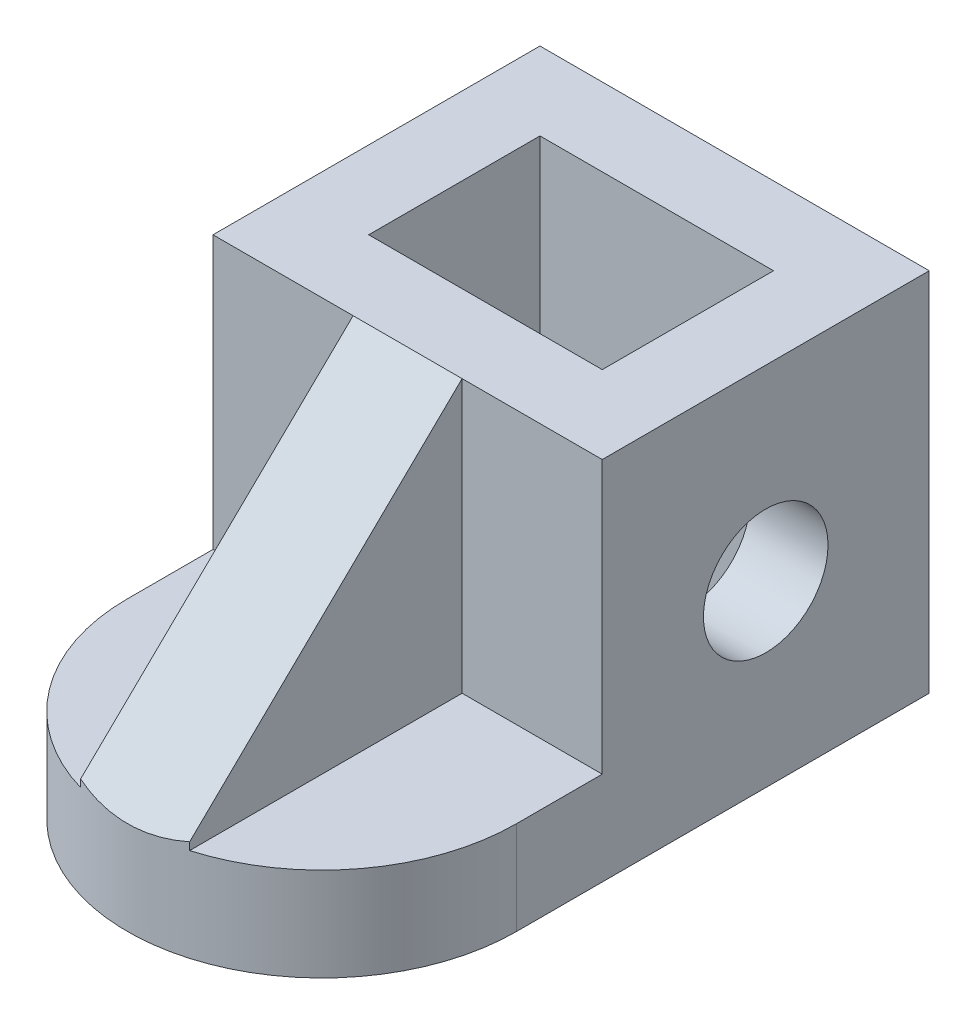
ISO-10303-21;
HEADER;
FILE_DESCRIPTION(('STEP AP214'),'2;1');
FILE_NAME('part.step','',(''),(''),'','','');
FILE_SCHEMA(('AUTOMOTIVE_DESIGN { 1 0 10303 214 1 1 1 1 }'));
ENDSEC;
DATA;
#1=APPLICATION_CONTEXT('core data for automotive mechanical design processes');
#2=APPLICATION_PROTOCOL_DEFINITION('international standard','automotive_design',2000,#1);
#3=PRODUCT_CONTEXT('',#1,'mechanical');
#4=PRODUCT('Part','Part','',(#3));
#5=PRODUCT_RELATED_PRODUCT_CATEGORY('part','',(#4));
#6=PRODUCT_DEFINITION_FORMATION('','',#4);
#7=PRODUCT_DEFINITION_CONTEXT('part definition',#1,'design');
#8=PRODUCT_DEFINITION('design','',#6,#7);
#9=PRODUCT_DEFINITION_SHAPE('','',#8);
#10=(LENGTH_UNIT() NAMED_UNIT(*) SI_UNIT(.MILLI.,.METRE.));
#11=(NAMED_UNIT(*) PLANE_ANGLE_UNIT() SI_UNIT($,.RADIAN.));
#12=(NAMED_UNIT(*) SI_UNIT($,.STERADIAN.) SOLID_ANGLE_UNIT());
#13=UNCERTAINTY_MEASURE_WITH_UNIT(LENGTH_MEASURE(1.E-05),#10,'distance_accuracy_value','');
#14=(GEOMETRIC_REPRESENTATION_CONTEXT(3) GLOBAL_UNCERTAINTY_ASSIGNED_CONTEXT((#13)) GLOBAL_UNIT_ASSIGNED_CONTEXT((#10,
#11,#12)) REPRESENTATION_CONTEXT('',''));
#15=CARTESIAN_POINT('',(0.,0.,0.));
#16=DIRECTION('',(0.,0.,1.));
#17=DIRECTION('',(1.,0.,0.));
#18=AXIS2_PLACEMENT_3D('',#15,#16,#17);
#19=CARTESIAN_POINT('',(-25.,6.,39.));
#20=DIRECTION('',(0.,-0.716994918814431,-0.697078393291808));
#21=DIRECTION('',(0.,0.697078393291808,-0.716994918814431));
#22=AXIS2_PLACEMENT_3D('',#19,#20,#21);
#23=PLANE('',#22);
#24=DIRECTION('',(0.,0.697078393291808,-0.716994918814431));
#25=VECTOR('',#24,1.);
#26=CARTESIAN_POINT('',(-32.,6.,39.));
#27=LINE('',#26,#25);
#28=CARTESIAN_POINT('',(-32.,6.97222222222222,38.));
#29=VERTEX_POINT('',#28);
#30=CARTESIAN_POINT('',(-32.,41.,3.00000000000002));
#31=VERTEX_POINT('',#30);
#32=EDGE_CURVE('E158',#29,#31,#27,.T.);
#33=ORIENTED_EDGE('',*,*,#32,.F.);
#34=CARTESIAN_POINT('',(-25.,30.3055555555556,14.));
#35=DIRECTION('',(0.,-0.716994918814431,-0.697078393291808));
#36=DIRECTION('',(0.,-0.697078393291808,0.716994918814431));
#37=AXIS2_PLACEMENT_3D('',#34,#35,#36);
#38=ELLIPSE('',#37,34.8677505850922,25.);
#39=CARTESIAN_POINT('',(-18.,6.97222222222222,38.));
#40=VERTEX_POINT('',#39);
#41=EDGE_CURVE('E145',#29,#40,#38,.F.);
#42=ORIENTED_EDGE('',*,*,#41,.T.);
#43=DIRECTION('',(0.,0.697078393291808,-0.716994918814431));
#44=VECTOR('',#43,1.);
#45=CARTESIAN_POINT('',(-18.,6.,39.));
#46=LINE('',#45,#44);
#47=CARTESIAN_POINT('',(-18.,41.,3.00000000000003));
#48=VERTEX_POINT('',#47);
#49=EDGE_CURVE('E53',#40,#48,#46,.T.);
#50=ORIENTED_EDGE('',*,*,#49,.T.);
#51=DIRECTION('',(1.,0.,0.));
#52=VECTOR('',#51,1.);
#53=CARTESIAN_POINT('',(-50.,41.,3.00000000000003));
#54=LINE('',#53,#52);
#55=EDGE_CURVE('E156',#31,#48,#54,.T.);
#56=ORIENTED_EDGE('',*,*,#55,.F.);
#57=EDGE_LOOP('',(#33,#42,#50,#56));
#58=FACE_BOUND('',#57,.T.);
#59=ADVANCED_FACE('F39',(#58),#23,.F.);
#60=CARTESIAN_POINT('',(-32.,17.5,0.));
#61=DIRECTION('',(1.,0.,0.));
#62=DIRECTION('',(0.,0.,-1.));
#63=AXIS2_PLACEMENT_3D('',#60,#61,#62);
#64=PLANE('',#63);
#65=DIRECTION('',(0.,-1.,0.));
#66=VECTOR('',#65,1.);
#67=CARTESIAN_POINT('',(-32.,14.,38.));
#68=LINE('',#67,#66);
#69=CARTESIAN_POINT('',(-32.,6.,38.));
#70=VERTEX_POINT('',#69);
#71=EDGE_CURVE('E143',#29,#70,#68,.T.);
#72=ORIENTED_EDGE('',*,*,#71,.F.);
#73=ORIENTED_EDGE('',*,*,#32,.T.);
#74=DIRECTION('',(0.,1.,0.));
#75=VECTOR('',#74,1.);
#76=CARTESIAN_POINT('',(-32.,5.99999999999999,3.00000000000003));
#77=LINE('',#76,#75);
#78=CARTESIAN_POINT('',(-32.,5.99999999999999,3.00000000000003));
#79=VERTEX_POINT('',#78);
#80=EDGE_CURVE('E165',#79,#31,#77,.T.);
#81=ORIENTED_EDGE('',*,*,#80,.F.);
#82=DIRECTION('',(0.,0.,-1.));
#83=VECTOR('',#82,1.);
#84=CARTESIAN_POINT('',(-32.,6.,39.));
#85=LINE('',#84,#83);
#86=EDGE_CURVE('E159',#70,#79,#85,.T.);
#87=ORIENTED_EDGE('',*,*,#86,.F.);
#88=EDGE_LOOP('',(#72,#73,#81,#87));
#89=FACE_BOUND('',#88,.T.);
#90=ADVANCED_FACE('F151',(#89),#64,.F.);
#91=CARTESIAN_POINT('',(-50.,-6.,39.));
#92=DIRECTION('',(0.,-1.,0.));
#93=DIRECTION('',(0.,0.,-1.));
#94=AXIS2_PLACEMENT_3D('',#91,#92,#93);
#95=PLANE('',#94);
#96=DIRECTION('',(-1.,0.,0.));
#97=VECTOR('',#96,1.);
#98=CARTESIAN_POINT('',(-40.,-6.,-29.));
#99=LINE('',#98,#97);
#100=CARTESIAN_POINT('',(-10.,-6.,-29.));
#101=VERTEX_POINT('',#100);
#102=CARTESIAN_POINT('',(-40.,-6.,-29.));
#103=VERTEX_POINT('',#102);
#104=EDGE_CURVE('E61',#101,#103,#99,.T.);
#105=ORIENTED_EDGE('',*,*,#104,.T.);
#106=DIRECTION('',(0.,0.,1.));
#107=VECTOR('',#106,1.);
#108=CARTESIAN_POINT('',(-40.,-6.,-29.));
#109=LINE('',#108,#107);
#110=CARTESIAN_POINT('',(-40.,-6.00000000000001,-6.99999999999997));
#111=VERTEX_POINT('',#110);
#112=EDGE_CURVE('E193',#103,#111,#109,.T.);
#113=ORIENTED_EDGE('',*,*,#112,.T.);
#114=DIRECTION('',(1.,0.,0.));
#115=VECTOR('',#114,1.);
#116=CARTESIAN_POINT('',(-40.,-6.00000000000001,-6.99999999999997));
#117=LINE('',#116,#115);
#118=CARTESIAN_POINT('',(-10.,-6.00000000000001,-6.99999999999997));
#119=VERTEX_POINT('',#118);
#120=EDGE_CURVE('E197',#111,#119,#117,.T.);
#121=ORIENTED_EDGE('',*,*,#120,.T.);
#122=DIRECTION('',(0.,0.,-1.));
#123=VECTOR('',#122,1.);
#124=CARTESIAN_POINT('',(-10.,-6.,-29.));
#125=LINE('',#124,#123);
#126=EDGE_CURVE('E188',#119,#101,#125,.T.);
#127=ORIENTED_EDGE('',*,*,#126,.T.);
#128=EDGE_LOOP('',(#105,#113,#121,#127));
#129=FACE_BOUND('',#128,.T.);
#130=DIRECTION('',(0.,0.,-1.));
#131=VECTOR('',#130,1.);
#132=CARTESIAN_POINT('',(0.,-6.,39.));
#133=LINE('',#132,#131);
#134=CARTESIAN_POINT('',(0.,-6.00000000000001,14.));
#135=VERTEX_POINT('',#134);
#136=CARTESIAN_POINT('',(0.,-6.,-39.));
#137=VERTEX_POINT('',#136);
#138=EDGE_CURVE('E245',#135,#137,#133,.T.);
#139=ORIENTED_EDGE('',*,*,#138,.F.);
#140=CARTESIAN_POINT('',(-25.,-6.00000000000001,14.));
#141=DIRECTION('',(0.,1.,0.));
#142=DIRECTION('',(0.,0.,1.));
#143=AXIS2_PLACEMENT_3D('',#140,#141,#142);
#144=CIRCLE('',#143,25.);
#145=CARTESIAN_POINT('',(-50.,-6.00000000000001,14.));
#146=VERTEX_POINT('',#145);
#147=EDGE_CURVE('E170',#146,#135,#144,.T.);
#148=ORIENTED_EDGE('',*,*,#147,.F.);
#149=DIRECTION('',(0.,0.,-1.));
#150=VECTOR('',#149,1.);
#151=CARTESIAN_POINT('',(-50.,-6.,39.));
#152=LINE('',#151,#150);
#153=CARTESIAN_POINT('',(-50.,-6.,-39.));
#154=VERTEX_POINT('',#153);
#155=EDGE_CURVE('E50',#146,#154,#152,.T.);
#156=ORIENTED_EDGE('',*,*,#155,.T.);
#157=DIRECTION('',(1.,0.,0.));
#158=VECTOR('',#157,1.);
#159=CARTESIAN_POINT('',(-50.,-6.,-39.));
#160=LINE('',#159,#158);
#161=EDGE_CURVE('E11',#154,#137,#160,.T.);
#162=ORIENTED_EDGE('',*,*,#161,.T.);
#163=EDGE_LOOP('',(#139,#148,#156,#162));
#164=FACE_BOUND('',#163,.T.);
#165=ADVANCED_FACE('F257',(#129,#164),#95,.T.);
#166=CARTESIAN_POINT('',(-18.,17.5,0.));
#167=DIRECTION('',(1.,0.,0.));
#168=DIRECTION('',(0.,0.,-1.));
#169=AXIS2_PLACEMENT_3D('',#166,#167,#168);
#170=PLANE('',#169);
#171=ORIENTED_EDGE('',*,*,#49,.F.);
#172=DIRECTION('',(0.,-1.,0.));
#173=VECTOR('',#172,1.);
#174=CARTESIAN_POINT('',(-18.,14.,38.));
#175=LINE('',#174,#173);
#176=CARTESIAN_POINT('',(-18.,6.,38.));
#177=VERTEX_POINT('',#176);
#178=EDGE_CURVE('E150',#40,#177,#175,.T.);
#179=ORIENTED_EDGE('',*,*,#178,.T.);
#180=DIRECTION('',(0.,0.,-1.));
#181=VECTOR('',#180,1.);
#182=CARTESIAN_POINT('',(-18.,6.,39.));
#183=LINE('',#182,#181);
#184=CARTESIAN_POINT('',(-18.,5.99999999999999,3.00000000000003));
#185=VERTEX_POINT('',#184);
#186=EDGE_CURVE('E174',#177,#185,#183,.T.);
#187=ORIENTED_EDGE('',*,*,#186,.T.);
#188=DIRECTION('',(0.,1.,0.));
#189=VECTOR('',#188,1.);
#190=CARTESIAN_POINT('',(-18.,5.99999999999999,3.00000000000003));
#191=LINE('',#190,#189);
#192=EDGE_CURVE('E173',#185,#48,#191,.T.);
#193=ORIENTED_EDGE('',*,*,#192,.T.);
#194=EDGE_LOOP('',(#171,#179,#187,#193));
#195=FACE_BOUND('',#194,.T.);
#196=ADVANCED_FACE('F293',(#195),#170,.T.);
#197=CARTESIAN_POINT('',(-50.,6.,39.));
#198=DIRECTION('',(0.,1.,0.));
#199=DIRECTION('',(0.,0.,1.));
#200=AXIS2_PLACEMENT_3D('',#197,#198,#199);
#201=PLANE('',#200);
#202=DIRECTION('',(0.,0.,1.));
#203=VECTOR('',#202,1.);
#204=CARTESIAN_POINT('',(-50.,6.,39.));
#205=LINE('',#204,#203);
#206=CARTESIAN_POINT('',(-50.,6.,3.00000000000003));
#207=VERTEX_POINT('',#206);
#208=CARTESIAN_POINT('',(-50.,6.,14.));
#209=VERTEX_POINT('',#208);
#210=EDGE_CURVE('E241',#207,#209,#205,.T.);
#211=ORIENTED_EDGE('',*,*,#210,.T.);
#212=CARTESIAN_POINT('',(-25.,6.,14.));
#213=DIRECTION('',(0.,1.,0.));
#214=DIRECTION('',(0.,0.,1.));
#215=AXIS2_PLACEMENT_3D('',#212,#213,#214);
#216=CIRCLE('',#215,25.);
#217=EDGE_CURVE('E288',#209,#70,#216,.T.);
#218=ORIENTED_EDGE('',*,*,#217,.T.);
#219=ORIENTED_EDGE('',*,*,#86,.T.);
#220=DIRECTION('',(1.,0.,0.));
#221=VECTOR('',#220,1.);
#222=CARTESIAN_POINT('',(-50.,5.99999999999999,3.00000000000003));
#223=LINE('',#222,#221);
#224=EDGE_CURVE('E230',#207,#79,#223,.T.);
#225=ORIENTED_EDGE('',*,*,#224,.F.);
#226=EDGE_LOOP('',(#211,#218,#219,#225));
#227=FACE_BOUND('',#226,.T.);
#228=ADVANCED_FACE('F291',(#227),#201,.T.);
#229=ORIENTED_EDGE('',*,*,#186,.F.);
#230=CARTESIAN_POINT('',(-25.,6.,14.));
#231=DIRECTION('',(0.,1.,0.));
#232=DIRECTION('',(0.,0.,1.));
#233=AXIS2_PLACEMENT_3D('',#230,#231,#232);
#234=CIRCLE('',#233,25.);
#235=CARTESIAN_POINT('',(0.,6.,14.));
#236=VERTEX_POINT('',#235);
#237=EDGE_CURVE('E147',#177,#236,#234,.T.);
#238=ORIENTED_EDGE('',*,*,#237,.T.);
#239=DIRECTION('',(0.,0.,1.));
#240=VECTOR('',#239,1.);
#241=CARTESIAN_POINT('',(0.,6.,39.));
#242=LINE('',#241,#240);
#243=CARTESIAN_POINT('',(0.,5.99999999999999,3.00000000000003));
#244=VERTEX_POINT('',#243);
#245=EDGE_CURVE('E247',#244,#236,#242,.T.);
#246=ORIENTED_EDGE('',*,*,#245,.F.);
#247=EDGE_CURVE('E231',#185,#244,#223,.T.);
#248=ORIENTED_EDGE('',*,*,#247,.F.);
#249=EDGE_LOOP('',(#229,#238,#246,#248));
#250=FACE_BOUND('',#249,.T.);
#251=ADVANCED_FACE('F281',(#250),#201,.T.);
#252=CARTESIAN_POINT('',(-50.,0.,0.));
#253=DIRECTION('',(-1.,0.,0.));
#254=DIRECTION('',(0.,0.,1.));
#255=AXIS2_PLACEMENT_3D('',#252,#253,#254);
#256=PLANE('',#255);
#257=CARTESIAN_POINT('',(-50.,17.,-18.));
#258=DIRECTION('',(-1.,0.,0.));
#259=DIRECTION('',(0.,0.,1.));
#260=AXIS2_PLACEMENT_3D('',#257,#258,#259);
#261=CIRCLE('',#260,8.);
#262=CARTESIAN_POINT('',(-50.,17.,-9.99999999999997));
#263=VERTEX_POINT('',#262);
#264=EDGE_CURVE('E180',#263,#263,#261,.T.);
#265=ORIENTED_EDGE('',*,*,#264,.F.);
#266=EDGE_LOOP('',(#265));
#267=FACE_BOUND('',#266,.T.);
#268=ORIENTED_EDGE('',*,*,#155,.F.);
#269=DIRECTION('',(0.,1.,0.));
#270=VECTOR('',#269,1.);
#271=CARTESIAN_POINT('',(-50.,-6.00000000000001,14.));
#272=LINE('',#271,#270);
#273=EDGE_CURVE('E162',#146,#209,#272,.T.);
#274=ORIENTED_EDGE('',*,*,#273,.T.);
#275=ORIENTED_EDGE('',*,*,#210,.F.);
#276=DIRECTION('',(0.,-1.,0.));
#277=VECTOR('',#276,1.);
#278=CARTESIAN_POINT('',(-50.,5.99999999999999,3.00000000000003));
#279=LINE('',#278,#277);
#280=CARTESIAN_POINT('',(-50.,41.,3.00000000000003));
#281=VERTEX_POINT('',#280);
#282=EDGE_CURVE('E218',#281,#207,#279,.T.);
#283=ORIENTED_EDGE('',*,*,#282,.F.);
#284=DIRECTION('',(0.,0.,1.));
#285=VECTOR('',#284,1.);
#286=CARTESIAN_POINT('',(-50.,41.,-39.));
#287=LINE('',#286,#285);
#288=CARTESIAN_POINT('',(-50.,41.,-39.));
#289=VERTEX_POINT('',#288);
#290=EDGE_CURVE('E220',#289,#281,#287,.T.);
#291=ORIENTED_EDGE('',*,*,#290,.F.);
#292=DIRECTION('',(0.,1.,0.));
#293=VECTOR('',#292,1.);
#294=CARTESIAN_POINT('',(-50.,-6.,-39.));
#295=LINE('',#294,#293);
#296=EDGE_CURVE('E237',#154,#289,#295,.T.);
#297=ORIENTED_EDGE('',*,*,#296,.F.);
#298=EDGE_LOOP('',(#268,#274,#275,#283,#291,#297));
#299=FACE_BOUND('',#298,.T.);
#300=ADVANCED_FACE('F266',(#267,#299),#256,.T.);
#301=CARTESIAN_POINT('',(0.,0.,0.));
#302=DIRECTION('',(-1.,0.,0.));
#303=DIRECTION('',(0.,0.,1.));
#304=AXIS2_PLACEMENT_3D('',#301,#302,#303);
#305=PLANE('',#304);
#306=CARTESIAN_POINT('',(0.,17.,-18.));
#307=DIRECTION('',(1.,0.,0.));
#308=DIRECTION('',(0.,0.,-1.));
#309=AXIS2_PLACEMENT_3D('',#306,#307,#308);
#310=CIRCLE('',#309,8.);
#311=CARTESIAN_POINT('',(0.,17.,-26.));
#312=VERTEX_POINT('',#311);
#313=EDGE_CURVE('E181',#312,#312,#310,.T.);
#314=ORIENTED_EDGE('',*,*,#313,.F.);
#315=EDGE_LOOP('',(#314));
#316=FACE_BOUND('',#315,.T.);
#317=DIRECTION('',(0.,1.,0.));
#318=VECTOR('',#317,1.);
#319=CARTESIAN_POINT('',(0.,-6.00000000000001,14.));
#320=LINE('',#319,#318);
#321=EDGE_CURVE('E259',#135,#236,#320,.T.);
#322=ORIENTED_EDGE('',*,*,#321,.F.);
#323=ORIENTED_EDGE('',*,*,#138,.T.);
#324=DIRECTION('',(0.,1.,0.));
#325=VECTOR('',#324,1.);
#326=CARTESIAN_POINT('',(0.,-6.,-39.));
#327=LINE('',#326,#325);
#328=CARTESIAN_POINT('',(0.,41.,-39.));
#329=VERTEX_POINT('',#328);
#330=EDGE_CURVE('E235',#137,#329,#327,.T.);
#331=ORIENTED_EDGE('',*,*,#330,.T.);
#332=DIRECTION('',(0.,0.,1.));
#333=VECTOR('',#332,1.);
#334=CARTESIAN_POINT('',(0.,41.,-39.));
#335=LINE('',#334,#333);
#336=CARTESIAN_POINT('',(0.,41.,3.00000000000003));
#337=VERTEX_POINT('',#336);
#338=EDGE_CURVE('E209',#329,#337,#335,.T.);
#339=ORIENTED_EDGE('',*,*,#338,.T.);
#340=DIRECTION('',(0.,-1.,0.));
#341=VECTOR('',#340,1.);
#342=CARTESIAN_POINT('',(0.,5.99999999999999,3.00000000000003));
#343=LINE('',#342,#341);
#344=EDGE_CURVE('E223',#337,#244,#343,.T.);
#345=ORIENTED_EDGE('',*,*,#344,.T.);
#346=ORIENTED_EDGE('',*,*,#245,.T.);
#347=EDGE_LOOP('',(#322,#323,#331,#339,#345,#346));
#348=FACE_BOUND('',#347,.T.);
#349=ADVANCED_FACE('F254',(#316,#348),#305,.F.);
#350=CARTESIAN_POINT('',(-50.,5.99999999999999,3.00000000000003));
#351=DIRECTION('',(0.,0.,1.));
#352=DIRECTION('',(0.,-1.,0.));
#353=AXIS2_PLACEMENT_3D('',#350,#351,#352);
#354=PLANE('',#353);
#355=ORIENTED_EDGE('',*,*,#224,.T.);
#356=ORIENTED_EDGE('',*,*,#80,.T.);
#357=EDGE_CURVE('E234',#281,#31,#54,.T.);
#358=ORIENTED_EDGE('',*,*,#357,.F.);
#359=ORIENTED_EDGE('',*,*,#282,.T.);
#360=EDGE_LOOP('',(#355,#356,#358,#359));
#361=FACE_BOUND('',#360,.T.);
#362=ADVANCED_FACE('F271',(#361),#354,.T.);
#363=CARTESIAN_POINT('',(-50.,-6.,-39.));
#364=DIRECTION('',(0.,0.,-1.));
#365=DIRECTION('',(-1.,0.,0.));
#366=AXIS2_PLACEMENT_3D('',#363,#364,#365);
#367=PLANE('',#366);
#368=ORIENTED_EDGE('',*,*,#330,.F.);
#369=ORIENTED_EDGE('',*,*,#161,.F.);
#370=ORIENTED_EDGE('',*,*,#296,.T.);
#371=DIRECTION('',(1.,0.,0.));
#372=VECTOR('',#371,1.);
#373=CARTESIAN_POINT('',(-50.,41.,-39.));
#374=LINE('',#373,#372);
#375=EDGE_CURVE('E225',#289,#329,#374,.T.);
#376=ORIENTED_EDGE('',*,*,#375,.T.);
#377=EDGE_LOOP('',(#368,#369,#370,#376));
#378=FACE_BOUND('',#377,.T.);
#379=ADVANCED_FACE('F41',(#378),#367,.T.);
#380=ORIENTED_EDGE('',*,*,#192,.F.);
#381=ORIENTED_EDGE('',*,*,#247,.T.);
#382=ORIENTED_EDGE('',*,*,#344,.F.);
#383=EDGE_CURVE('E240',#48,#337,#54,.T.);
#384=ORIENTED_EDGE('',*,*,#383,.F.);
#385=EDGE_LOOP('',(#380,#381,#382,#384));
#386=FACE_BOUND('',#385,.T.);
#387=ADVANCED_FACE('F280',(#386),#354,.T.);
#388=CARTESIAN_POINT('',(-50.,41.,-39.));
#389=DIRECTION('',(0.,1.,0.));
#390=DIRECTION('',(0.,0.,1.));
#391=AXIS2_PLACEMENT_3D('',#388,#389,#390);
#392=PLANE('',#391);
#393=DIRECTION('',(0.,0.,-1.));
#394=VECTOR('',#393,1.);
#395=CARTESIAN_POINT('',(-10.,41.,-29.));
#396=LINE('',#395,#394);
#397=CARTESIAN_POINT('',(-10.,41.,-6.99999999999996));
#398=VERTEX_POINT('',#397);
#399=CARTESIAN_POINT('',(-10.,41.,-29.));
#400=VERTEX_POINT('',#399);
#401=EDGE_CURVE('E190',#398,#400,#396,.T.);
#402=ORIENTED_EDGE('',*,*,#401,.F.);
#403=DIRECTION('',(1.,0.,0.));
#404=VECTOR('',#403,1.);
#405=CARTESIAN_POINT('',(-40.,41.,-6.99999999999996));
#406=LINE('',#405,#404);
#407=CARTESIAN_POINT('',(-40.,41.,-6.99999999999996));
#408=VERTEX_POINT('',#407);
#409=EDGE_CURVE('E191',#408,#398,#406,.T.);
#410=ORIENTED_EDGE('',*,*,#409,.F.);
#411=DIRECTION('',(0.,0.,1.));
#412=VECTOR('',#411,1.);
#413=CARTESIAN_POINT('',(-40.,41.,-29.));
#414=LINE('',#413,#412);
#415=CARTESIAN_POINT('',(-40.,41.,-29.));
#416=VERTEX_POINT('',#415);
#417=EDGE_CURVE('E204',#416,#408,#414,.T.);
#418=ORIENTED_EDGE('',*,*,#417,.F.);
#419=DIRECTION('',(-1.,0.,0.));
#420=VECTOR('',#419,1.);
#421=CARTESIAN_POINT('',(-40.,41.,-29.));
#422=LINE('',#421,#420);
#423=EDGE_CURVE('E198',#400,#416,#422,.T.);
#424=ORIENTED_EDGE('',*,*,#423,.F.);
#425=EDGE_LOOP('',(#402,#410,#418,#424));
#426=FACE_BOUND('',#425,.T.);
#427=ORIENTED_EDGE('',*,*,#55,.T.);
#428=ORIENTED_EDGE('',*,*,#383,.T.);
#429=ORIENTED_EDGE('',*,*,#338,.F.);
#430=ORIENTED_EDGE('',*,*,#375,.F.);
#431=ORIENTED_EDGE('',*,*,#290,.T.);
#432=ORIENTED_EDGE('',*,*,#357,.T.);
#433=EDGE_LOOP('',(#427,#428,#429,#430,#431,#432));
#434=FACE_BOUND('',#433,.T.);
#435=ADVANCED_FACE('F269',(#426,#434),#392,.T.);
#436=CARTESIAN_POINT('',(-10.,-6.,-29.));
#437=DIRECTION('',(1.,0.,0.));
#438=DIRECTION('',(0.,0.,-1.));
#439=AXIS2_PLACEMENT_3D('',#436,#437,#438);
#440=PLANE('',#439);
#441=CARTESIAN_POINT('',(-10.,17.,-18.));
#442=DIRECTION('',(1.,0.,0.));
#443=DIRECTION('',(0.,0.,-1.));
#444=AXIS2_PLACEMENT_3D('',#441,#442,#443);
#445=CIRCLE('',#444,8.);
#446=CARTESIAN_POINT('',(-10.,17.,-26.));
#447=VERTEX_POINT('',#446);
#448=EDGE_CURVE('E183',#447,#447,#445,.T.);
#449=ORIENTED_EDGE('',*,*,#448,.T.);
#450=EDGE_LOOP('',(#449));
#451=FACE_BOUND('',#450,.T.);
#452=ORIENTED_EDGE('',*,*,#401,.T.);
#453=DIRECTION('',(0.,1.,0.));
#454=VECTOR('',#453,1.);
#455=CARTESIAN_POINT('',(-10.,-6.,-29.));
#456=LINE('',#455,#454);
#457=EDGE_CURVE('E199',#101,#400,#456,.T.);
#458=ORIENTED_EDGE('',*,*,#457,.F.);
#459=ORIENTED_EDGE('',*,*,#126,.F.);
#460=DIRECTION('',(0.,1.,0.));
#461=VECTOR('',#460,1.);
#462=CARTESIAN_POINT('',(-10.,-6.00000000000001,-6.99999999999997));
#463=LINE('',#462,#461);
#464=EDGE_CURVE('E207',#119,#398,#463,.T.);
#465=ORIENTED_EDGE('',*,*,#464,.T.);
#466=EDGE_LOOP('',(#452,#458,#459,#465));
#467=FACE_BOUND('',#466,.T.);
#468=ADVANCED_FACE('F325',(#451,#467),#440,.F.);
#469=CARTESIAN_POINT('',(-40.,-6.00000000000001,-6.99999999999997));
#470=DIRECTION('',(0.,0.,1.));
#471=DIRECTION('',(0.,-1.,0.));
#472=AXIS2_PLACEMENT_3D('',#469,#470,#471);
#473=PLANE('',#472);
#474=ORIENTED_EDGE('',*,*,#464,.F.);
#475=ORIENTED_EDGE('',*,*,#120,.F.);
#476=DIRECTION('',(0.,1.,0.));
#477=VECTOR('',#476,1.);
#478=CARTESIAN_POINT('',(-40.,-6.00000000000001,-6.99999999999997));
#479=LINE('',#478,#477);
#480=EDGE_CURVE('E208',#111,#408,#479,.T.);
#481=ORIENTED_EDGE('',*,*,#480,.T.);
#482=ORIENTED_EDGE('',*,*,#409,.T.);
#483=EDGE_LOOP('',(#474,#475,#481,#482));
#484=FACE_BOUND('',#483,.T.);
#485=ADVANCED_FACE('F316',(#484),#473,.F.);
#486=CARTESIAN_POINT('',(-40.,-6.,-29.));
#487=DIRECTION('',(-1.,0.,0.));
#488=DIRECTION('',(0.,0.,1.));
#489=AXIS2_PLACEMENT_3D('',#486,#487,#488);
#490=PLANE('',#489);
#491=CARTESIAN_POINT('',(-40.,17.,-18.));
#492=DIRECTION('',(-1.,0.,0.));
#493=DIRECTION('',(0.,0.,1.));
#494=AXIS2_PLACEMENT_3D('',#491,#492,#493);
#495=CIRCLE('',#494,8.);
#496=CARTESIAN_POINT('',(-40.,17.,-9.99999999999997));
#497=VERTEX_POINT('',#496);
#498=EDGE_CURVE('E178',#497,#497,#495,.T.);
#499=ORIENTED_EDGE('',*,*,#498,.T.);
#500=EDGE_LOOP('',(#499));
#501=FACE_BOUND('',#500,.T.);
#502=ORIENTED_EDGE('',*,*,#417,.T.);
#503=ORIENTED_EDGE('',*,*,#480,.F.);
#504=ORIENTED_EDGE('',*,*,#112,.F.);
#505=DIRECTION('',(0.,1.,0.));
#506=VECTOR('',#505,1.);
#507=CARTESIAN_POINT('',(-40.,-6.,-29.));
#508=LINE('',#507,#506);
#509=EDGE_CURVE('E211',#103,#416,#508,.T.);
#510=ORIENTED_EDGE('',*,*,#509,.T.);
#511=EDGE_LOOP('',(#502,#503,#504,#510));
#512=FACE_BOUND('',#511,.T.);
#513=ADVANCED_FACE('F321',(#501,#512),#490,.F.);
#514=CARTESIAN_POINT('',(-40.,-6.,-29.));
#515=DIRECTION('',(0.,0.,-1.));
#516=DIRECTION('',(0.,1.,0.));
#517=AXIS2_PLACEMENT_3D('',#514,#515,#516);
#518=PLANE('',#517);
#519=ORIENTED_EDGE('',*,*,#423,.T.);
#520=ORIENTED_EDGE('',*,*,#509,.F.);
#521=ORIENTED_EDGE('',*,*,#104,.F.);
#522=ORIENTED_EDGE('',*,*,#457,.T.);
#523=EDGE_LOOP('',(#519,#520,#521,#522));
#524=FACE_BOUND('',#523,.T.);
#525=ADVANCED_FACE('F320',(#524),#518,.F.);
#526=CARTESIAN_POINT('',(-10.,17.,-18.));
#527=DIRECTION('',(1.,0.,0.));
#528=DIRECTION('',(0.,0.,-1.));
#529=AXIS2_PLACEMENT_3D('',#526,#527,#528);
#530=CYLINDRICAL_SURFACE('',#529,8.);
#531=ORIENTED_EDGE('',*,*,#448,.F.);
#532=EDGE_LOOP('',(#531));
#533=FACE_BOUND('',#532,.T.);
#534=ORIENTED_EDGE('',*,*,#313,.T.);
#535=EDGE_LOOP('',(#534));
#536=FACE_BOUND('',#535,.T.);
#537=ADVANCED_FACE('F312',(#533,#536),#530,.F.);
#538=CARTESIAN_POINT('',(-40.,17.,-18.));
#539=DIRECTION('',(-1.,0.,0.));
#540=DIRECTION('',(0.,0.,1.));
#541=AXIS2_PLACEMENT_3D('',#538,#539,#540);
#542=CYLINDRICAL_SURFACE('',#541,8.);
#543=ORIENTED_EDGE('',*,*,#498,.F.);
#544=EDGE_LOOP('',(#543));
#545=FACE_BOUND('',#544,.T.);
#546=ORIENTED_EDGE('',*,*,#264,.T.);
#547=EDGE_LOOP('',(#546));
#548=FACE_BOUND('',#547,.T.);
#549=ADVANCED_FACE('F309',(#545,#548),#542,.F.);
#550=CARTESIAN_POINT('',(-25.,-6.00000000000001,14.));
#551=DIRECTION('',(0.,1.,0.));
#552=DIRECTION('',(0.,0.,1.));
#553=AXIS2_PLACEMENT_3D('',#550,#551,#552);
#554=CYLINDRICAL_SURFACE('',#553,25.);
#555=ORIENTED_EDGE('',*,*,#147,.T.);
#556=ORIENTED_EDGE('',*,*,#321,.T.);
#557=ORIENTED_EDGE('',*,*,#237,.F.);
#558=ORIENTED_EDGE('',*,*,#178,.F.);
#559=ORIENTED_EDGE('',*,*,#41,.F.);
#560=ORIENTED_EDGE('',*,*,#71,.T.);
#561=ORIENTED_EDGE('',*,*,#217,.F.);
#562=ORIENTED_EDGE('',*,*,#273,.F.);
#563=EDGE_LOOP('',(#555,#556,#557,#558,#559,#560,#561,#562));
#564=FACE_BOUND('',#563,.T.);
#565=ADVANCED_FACE('F144',(#564),#554,.T.);
#566=CLOSED_SHELL('',(#59,#90,#165,#196,#228,#251,#300,#349,#362,#379,#387,#435,#468,#485,#513,
#525,#537,#549,#565));
#567=MANIFOLD_SOLID_BREP('B2',#566);
#568=ADVANCED_BREP_SHAPE_REPRESENTATION('',(#18,#567),#14);
#569=SHAPE_DEFINITION_REPRESENTATION(#9,#568);
ENDSEC;
END-ISO-10303-21;
